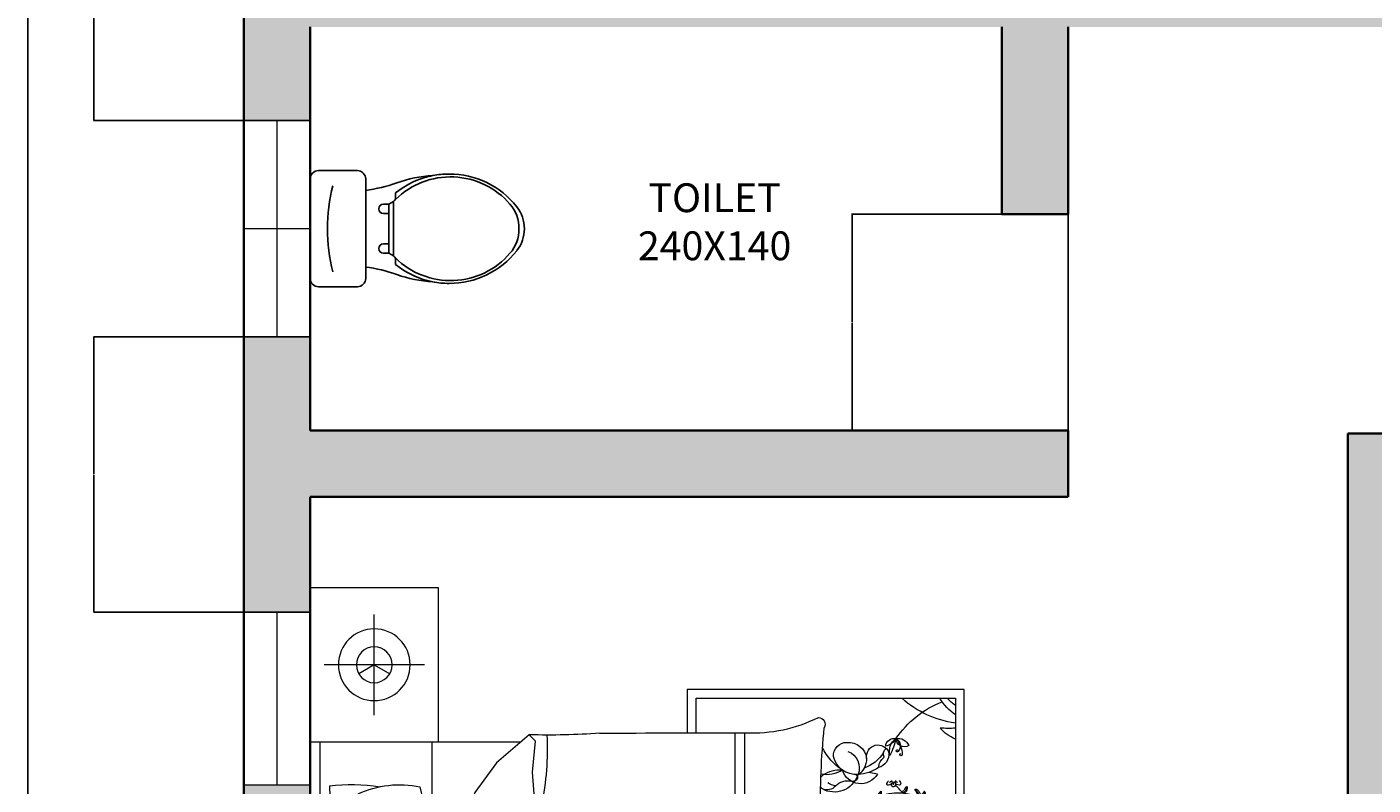
# Model space of a CAD drawing. Units: centimetres. Extents: x 2178 to 3635, y 1064 to 2635.
# Tile 2 of 9: x 2178 to 2645, y 1502 to 1765. Entities that reach past the tile are written whole.
import ezdxf

# ---------------------------------------------------------------- set-up
doc = ezdxf.new("R2010")
doc.units = ezdxf.units.CM
for name, color, linetype, lineweight in [('A-ANNO-DIMS', 2, 'Continuous', 18), ('A-AREA-IDEN', 7, 'Continuous', 18), ('A-DOOR', 32, 'Continuous', 25), ('A-FLOR-FIXT', 42, 'Continuous', 18), ('A-FURN', 42, 'Continuous', 18), ('A-GLAZ', 4, 'Continuous', 18), ('A-WALL', 7, 'Continuous', 35)]:
    doc.layers.add(name, color=color, linetype=linetype, lineweight=lineweight)
doc.layers.add('A-WALL-PATT', color=18, linetype='Continuous', lineweight=13, true_color=0x000000)
doc.layers.add('WC-Detail_dwgmodels.com', color=251, linetype='Continuous')
doc.layers.add('WC-Outline_dwgmodels.com', color=250, linetype='Continuous')
doc.styles.get("Standard").update_dxf_attribs({"font": 'arial.ttf'})
doc.dimstyles.get("Standard").update_dxf_attribs({"dimtxt": 0.18, "dimasz": 0.18, "dimexe": 0.18, "dimexo": 0.0625, "dimgap": 0.09, "dimtad": 0, "dimtih": 1, "dimtoh": 1, "dimdec": 4, "dimzin": 0, "dimdsep": 46, "dimtxsty": 'Standard', "dimcen": 0.09, "dimadec": 0, "dimazin": 0, "dimtfac": 1, "dimtdec": 4, "dimtofl": 0, "dimtmove": 0, "dimatfit": 3, "dimfxl": 1, "dimtolj": 1, "dimtzin": 0, "dimarcsym": 0})

# ---------------------------------------------------------------- blocks, each defined once
blk = doc.blocks.new('bed')
for p, q in [((2798.77, 2937.13), (3098.77, 2937.13)), ((2858.77, 2937.13), (2858.77, 2854.79)), ((2828.77, 2892.53), (2828.77, 2931.73)), ((3038.77, 2933.28), (2858.77, 2933.28)), ((3068.77, 2892.53), (3068.77, 2931.73)), ((2848.37, 2912.13), (2809.17, 2912.13)), ((3049.17, 2912.13), (3088.37, 2912.13)), ((2858.77, 2889.72), (3038.77, 2889.72)), ((2900.44, 2880.8), (2933.16, 2889.72)), ((2941.19, 2889.72), (2924.75, 2866.84)), ((2878.57, 2872.91), (2900.44, 2880.8)), ((2867.02, 2864.41), (2878.57, 2872.91)), ((3037.85, 2874.18), (2928.92, 2872.64)), ((3037.97, 2877.26), (2931.16, 2875.76)), ((2924.75, 2866.84), (2918.06, 2849.23)), ((2856.09, 2851.66), (2867.02, 2864.41)), ((3037.71, 2861.65), (2922.6, 2861.18)), ((3037.69, 2864.73), (2923.78, 2864.28)), ((2858.52, 2849.23), (2856.09, 2851.66)), ((2870.67, 2850.44), (2858.52, 2849.23)), ((2885.86, 2849.23), (2870.67, 2850.44)), ((2899.23, 2847.41), (2885.86, 2849.23)), ((2907.13, 2843.76), (2899.23, 2847.41)), ((2918.06, 2849.23), (2916.85, 2841.33)), ((2916.85, 2841.33), (2907.13, 2843.76)), ((2838.37, 2790.07), (2855.34, 2790.07)), ((2838.37, 2682), (2838.37, 2790.07)), ((3040.44, 2790.07), (3057.08, 2790.07)), ((3057.08, 2790.07), (3057.08, 2682)), ((2855.33, 2786.59), (2841.85, 2786.59)), ((2841.85, 2786.59), (2841.85, 2685.48)), ((3053.6, 2786.59), (3040.38, 2786.59)), ((3053.6, 2685.48), (3053.6, 2786.59)), ((3040.42, 2767.62), (2855.31, 2767.62)), ((3040.13, 2771.36), (2855.32, 2771.36)), ((3009.67, 2738.15), (2887.87, 2738.15)), ((2871.41, 2715.89), (2870.75, 2719.28)), ((2892.38, 2715.89), (2893.04, 2719.28)), ((3003.07, 2715.89), (3002.41, 2719.28)), ((3024.04, 2715.89), (3024.7, 2719.28)), ((2841.85, 2685.48), (3053.6, 2685.48)), ((3057.08, 2682), (2838.37, 2682))]:
    blk.add_line(p, q)
for points in [[(2858.77, 2887.13), (2798.77, 2887.13), (2798.77, 2937.13)], [(3038.77, 2937.13), (3038.77, 2887.13), (3098.77, 2887.13), (3098.77, 2937.13)], [(2828.77, 2912.13), (2832.27, 2918.19)], [(3068.77, 2912.13), (3065.27, 2918.19)], [(2828.77, 2912.13), (2832.27, 2906.07)], [(3068.77, 2912.13), (3065.27, 2906.07)]]:
    blk.add_lwpolyline(points)
for points in [[(2876, 2929.65, 0.074897), (2876.37, 2910.06, -0.472817)], [(2947.37, 2908.96, 0.14099), (2947.97, 2928.95, 0.235245)], [(2960.18, 2908.96, -0.14099), (2959.58, 2928.95, -0.235245)], [(3021.54, 2929.65, -0.074897), (3021.18, 2910.06, 0.472817)], [(2855.46, 2824.19, 0.001242), (2855.31, 2767.26, -0.127202), (2849.3, 2738.9)], [(3040.05, 2773.72, 0.056112), (3042.23, 2757.21, 0.095341), (3046.45, 2741.32)]]:
    blk.add_lwpolyline(points, format="xyb")
for centre, radius in [((2828.77, 2912.13), 14), ((3068.77, 2912.13), 14), ((2828.77, 2912.13), 7), ((3068.77, 2912.13), 7), ((2888.74, 2705.02), 0.764), ((3006.71, 2705.02), 0.764), ((2883.74, 2696.97), 0.764), ((3011.71, 2696.97), 0.764)]:
    blk.add_circle(centre, radius)
for centre, radius, start, end in [((2917.11, 2821.09), 108.8, 82.2196, 99.497), ((2985.93, 2877.16), 52.74, 76.3427, 101.1841), ((3041.36, 5784.66), 2859.79, 266.68521, 267.14978), ((2940.09, 2876.08), 53.46, 81.5249, 103.96), ((2963.69, 2914.69), 14.84, 63.3437, 106.1026), ((2856.18, 5784.66), 2859.79, 272.85022, 273.31479), ((2914.22, 2902.19), 38.67, 155.1316, 191.7583), ((2983.32, 2902.19), 38.67, 348.2417, 24.8684), ((2912, 2898.93), 36.76, 354.0129, 15.8293), ((2995.54, 2898.93), 36.76, 164.1707, 185.9871), ((2886.7, 2933.16), 40.2, 255.1039, 281.0369), ((2907.87, 2961.74), 69.73, 258.0397, 289.2615), ((2936.1, 2946.52), 52.9, 259.8617, 283.6238), ((2965.7, 2909.52), 15.9, 245.0183, 288.5407), ((2993.49, 2930.2), 38.19, 243.8761, 286.1746), ((3010.84, 2933.16), 40.2, 258.9631, 284.8961), ((3576.57, 2853.06), 539.05, 176.1, 180.9282), ((2581.02, 2844.2), 275.17, 355.8294, 1.553), ((2861.22, 2957.89), 113.22, 267.4519, 281.3392), ((2888.28, 2822.94), 24.42, 66.2616, 101.3392), ((2937.68, 2954.7), 116.34, 250.1194, 259.3383), ((2916.17, 2841.09), 0.724, 268.8623, 19.7536), ((3740.68, 2833.46), 703.17, 179.11454, 184.87351), ((3044.17, 2739.79), 2.73, 246.5219, 33.8264), ((2852.06, 2739.09), 2.77, 183.98, 297.3412), ((2884.29, 2425.86), 312.3, 89.3433, 95.6887), ((2850.89, 2717.02), 22.71, 33.6671, 63.2997), ((2881.32, 2730.53), 11.57, 145.785, 184.7304), ((2859.22, 2735.93), 12.43, 328.8218, 9.1554), ((2874.61, 2734.83), 3.61, 120.0293, 142.325), ((2868.85, 2732.7), 9.56, 289.2822, 29.1751), ((2873.09, 2735.54), 4.49, 311.5653, 23.8354), ((2874.61, 2734.83), 3.61, 44.4517, 63.558), ((2894.94, 2732.7), 9.56, 150.8249, 250.7178), ((2890.7, 2735.54), 4.49, 156.1646, 228.4347), ((2889.17, 2734.83), 3.61, 113.229, 135.5483), ((2889.17, 2734.83), 3.61, 37.675, 66.7144), ((2882.46, 2730.53), 11.57, 355.2696, 34.215), ((2904.56, 2735.93), 12.43, 169.7133, 211.1782), ((2912.89, 2717.02), 22.71, 111.4941, 146.3329), ((2982.56, 2717.02), 22.71, 33.6671, 68.5059), ((3012.99, 2730.53), 11.57, 145.785, 184.7304), ((2990.89, 2735.93), 12.43, 328.8218, 10.2867), ((3006.28, 2734.83), 3.61, 113.2856, 142.325), ((3000.51, 2732.7), 9.56, 289.2822, 29.1751), ((3006.28, 2734.83), 3.61, 44.4517, 66.7144), ((3004.75, 2735.54), 4.49, 311.5653, 23.8354), ((3018.86, 2446.37), 291.92, 85.2402, 91.8035), ((3026.6, 2732.7), 9.56, 150.8249, 250.7178), ((3022.36, 2735.54), 4.49, 156.1646, 228.4347), ((3020.84, 2734.83), 3.61, 106.6343, 135.5483), ((3020.84, 2734.83), 3.61, 37.675, 72.5814), ((3014.13, 2730.53), 11.57, 355.2696, 34.215), ((3036.23, 2735.93), 12.43, 169.249, 211.1782), ((3044.56, 2717.02), 22.71, 113.6453, 146.3329), ((2864.12, 2727.92), 5.07, 84.4856, 181.0538), ((2862.56, 2724.18), 9.02, 355.2933, 76.921), ((2880.15, 2727.58), 6.15, 131.5653, 195.1471), ((2867.4, 2730.97), 8.62, 7.436, 29.9149), ((2883.64, 2727.58), 6.15, 344.8529, 48.4347), ((2896.38, 2730.97), 8.62, 150.0851, 172.564), ((2901.22, 2724.18), 9.02, 103.079, 184.7067), ((2899.66, 2727.92), 5.07, 358.9462, 95.5144), ((2995.79, 2727.92), 5.07, 84.4856, 181.0538), ((2994.23, 2724.18), 9.02, 355.2933, 76.921), ((3011.81, 2727.58), 6.15, 131.5653, 195.1471), ((2999.07, 2730.97), 8.62, 7.436, 29.9149), ((3015.3, 2727.58), 6.15, 344.8529, 48.4347), ((3028.05, 2730.97), 8.62, 150.0851, 172.564), ((3032.89, 2724.18), 9.02, 103.079, 184.7067), ((3031.33, 2727.92), 5.07, 358.9462, 95.5144), ((2866.2, 2727.2), 7.17, 174.9449, 262.8857), ((2869.01, 2729.92), 6.96, 201.5819, 291.4221), ((2867.69, 2722.36), 7.46, 299.9085, 73.1337), ((2872.41, 2725.49), 1.86, 257.3041, 15.1471), ((2896.09, 2722.36), 7.46, 106.8663, 240.0915), ((2891.37, 2725.49), 1.86, 164.8529, 282.6959), ((2894.77, 2729.92), 6.96, 248.5779, 338.4181), ((2897.59, 2727.2), 7.17, 277.1143, 5.0551), ((2997.86, 2727.2), 7.17, 174.9449, 262.8857), ((3000.68, 2729.92), 6.96, 201.5819, 291.4221), ((2999.36, 2722.36), 7.46, 299.9085, 73.1337), ((3004.08, 2725.49), 1.86, 257.3041, 15.1471), ((3027.76, 2722.36), 7.46, 106.8663, 240.0915), ((3023.04, 2725.49), 1.86, 164.8529, 282.6959), ((3026.44, 2729.92), 6.96, 248.5779, 338.4181), ((3029.25, 2727.2), 7.17, 277.1143, 5.0551), ((2864.55, 2715.65), 4.5, 80.264, 250.8688), ((2855.62, 2725.56), 14.16, 301.2614, 341.7045), ((2864.95, 2728.79), 8.71, 272.3591, 324.0401), ((2855.49, 2724.42), 16.1, 326.2883, 356.5076), ((2881.32, 2730.53), 11.57, 212.7011, 216.3445), ((2882.75, 2722.67), 0.578, 102.7051, 280.4384), ((2882.69, 2723.02), 0.94, 280.4384, 100.4136), ((2882.46, 2730.53), 11.57, 323.6555, 327.2989), ((2898.83, 2728.79), 8.71, 215.9599, 267.6409), ((2908.3, 2724.42), 16.1, 183.4924, 213.7117), ((2908.16, 2725.56), 14.16, 198.2955, 238.7386), ((2899.24, 2715.65), 4.5, 289.1312, 99.736), ((2951.17, 2718.35), 3.25, 63.0274, 163.8037), ((2947.89, 2725.94), 6.69, 271.4585, 315.3727), ((2954.28, 2718.35), 3.25, 16.1963, 116.9726), ((2957.56, 2725.94), 6.69, 224.6273, 268.5415), ((2996.21, 2715.65), 4.5, 80.264, 250.8688), ((2987.29, 2725.56), 14.16, 301.2614, 341.7045), ((2996.62, 2728.79), 8.71, 272.3591, 324.0401), ((2987.15, 2724.42), 16.1, 326.2883, 356.5076), ((3012.99, 2730.53), 11.57, 212.7011, 216.3445), ((3012.76, 2723.02), 0.94, 79.5864, 259.5616), ((3012.7, 2722.67), 0.578, 259.5616, 77.2949), ((3014.13, 2730.53), 11.57, 323.6555, 327.2989), ((3030.5, 2728.79), 8.71, 215.9599, 267.6409), ((3039.96, 2724.42), 16.1, 183.4924, 213.7117), ((3039.83, 2725.56), 14.16, 198.2955, 238.7386), ((3030.9, 2715.65), 4.5, 289.1312, 99.736), ((2863.47, 2717), 5.62, 265.969, 344.3045), ((2869.52, 2709.53), 5.99, 96.1662, 141.5825), ((2879.44, 2713.73), 1.58, 101.3256, 154.4621), ((2877.17, 2719.07), 4.74, 280.2588, 300.656), ((2903.55, 2707.57), 24.85, 163.5842, 183.8277), ((2876.15, 2719.06), 4.82, 308.2101, 316.3071), ((2879.11, 2715.89), 1.44, 278.3432, 4.2869), ((2878.31, 2717.16), 2.51, 300.656, 332.6341), ((2880.2, 2715.5), 0.611, 55.7657, 157.4417), ((2903.55, 2707.57), 24.85, 153.0032, 159.8941), ((2881.15, 2716.07), 0.611, 84.3784, 186.0543), ((2880.58, 2718.52), 2.51, 269.1859, 301.164), ((2881.32, 2717.22), 1.44, 237.5332, 323.4768), ((2879.92, 2721.32), 4.82, 285.5129, 293.6099), ((2883.07, 2715.9), 1.58, 87.3579, 140.4944), ((2879.43, 2720.42), 4.74, 301.164, 321.5612), ((2875.57, 2721.25), 8.46, 324.6898, 333.4936), ((2894.26, 2709.53), 5.99, 38.4175, 83.8338), ((2900.32, 2717), 5.62, 195.6955, 274.031), ((2951.1, 2680.2), 39.18, 94.4623, 172.255), ((2951.27, 2716.33), 4.34, 137.7873, 219.1145), ((2946.34, 2716.47), 3.27, 298.5391, 58.3627), ((2951.26, 2719.13), 3.2, 177.7585, 283.852), ((2950.61, 2713.61), 6.19, 45.5411, 114.3101), ((2956.25, 2745.4), 27.41, 252.593, 267.2582), ((2957.43, 2722.47), 9.91, 198.9159, 238.011), ((2954.84, 2713.61), 6.19, 65.6899, 134.4589), ((2949.2, 2745.4), 27.41, 272.7418, 287.407), ((2951.92, 2716.43), 0.424, 283.852, 219.9245), ((2952.44, 2714.47), 0.487, 238.011, 71.5592), ((2952.52, 2714.71), 0.236, 71.5592, 188.0167), ((2953.01, 2714.47), 0.487, 108.4408, 301.989), ((2952.93, 2714.71), 0.236, 351.9833, 108.4408), ((2953.49, 2716.59), 0.255, 320.1909, 256.0209), ((2948.02, 2722.47), 9.91, 301.989, 341.0841), ((2954.19, 2719.13), 3.2, 256.148, 2.2415), ((2959.11, 2716.47), 3.27, 121.6373, 241.4609), ((2954.18, 2716.33), 4.34, 320.8855, 42.2127), ((2953.08, 2689.24), 30.32, 352.8636, 81.8197), ((2995.13, 2717), 5.62, 265.969, 344.3045), ((3001.19, 2709.53), 5.99, 96.1662, 141.5825), ((3012.38, 2715.9), 1.58, 39.5056, 92.6421), ((3016.02, 2720.42), 4.74, 218.4388, 238.836), ((3019.88, 2721.25), 8.46, 206.5064, 215.3102), ((3014.13, 2717.22), 1.44, 216.5232, 302.4668), ((3014.87, 2718.52), 2.51, 238.836, 270.8141), ((3015.53, 2721.32), 4.82, 246.3901, 254.4871), ((2991.9, 2707.57), 24.85, 20.1059, 26.9968), ((3014.3, 2716.07), 0.611, 353.9457, 95.6216), ((3016.34, 2715.89), 1.44, 175.7131, 261.6568), ((3015.25, 2715.5), 0.611, 22.5583, 124.2343), ((3017.14, 2717.16), 2.51, 207.3659, 239.344), ((2991.9, 2707.57), 24.85, 356.1723, 16.4158), ((3019.3, 2719.06), 4.82, 223.6929, 231.7899), ((3018.28, 2719.07), 4.74, 239.344, 259.7412), ((3016.01, 2713.73), 1.58, 25.5379, 78.6744), ((3031.98, 2717), 5.62, 195.6955, 274.031), ((3025.93, 2709.53), 5.99, 38.4175, 83.8338), ((2860.73, 2709.42), 3.25, 92.9516, 193.728), ((2854.09, 2714.37), 6.69, 301.3827, 345.2969), ((2862.6, 2705.03), 6.19, 75.4653, 144.2343), ((2851.64, 2735.41), 27.41, 282.5173, 297.1824), ((2863.62, 2710.77), 2.76, 63.9755, 143.2681), ((2874.99, 2710.74), 1.27, 101.5637, 142.6358), ((2873.93, 2709.56), 0.764, 273.2768, 86.7232), ((2874.82, 2710.28), 0.73, 91.1081, 181.8675), ((2875.59, 2708.82), 1.58, 80.3487, 133.6538), ((2873.96, 2711.74), 1.84, 288.7263, 352.5032), ((2875.3, 2707.17), 2.5, 83.0852, 105.7171), ((2875.21, 2711.65), 0.59, 345.2356, 144.9248), ((2875.75, 2709.72), 0.658, 317.6792, 80.3487), ((2878.27, 2722.86), 8.46, 268.3264, 277.1302), ((2900.16, 2710.77), 2.76, 36.7319, 116.0245), ((2901.18, 2705.03), 6.19, 35.7657, 104.5347), ((2912.15, 2735.41), 27.41, 242.8176, 257.4827), ((2903.05, 2709.42), 3.25, 346.272, 87.0484), ((2909.69, 2714.37), 6.69, 194.7031, 238.6173), ((2992.4, 2709.42), 3.25, 92.9516, 193.728), ((2985.76, 2714.37), 6.69, 301.3827, 345.2969), ((2994.27, 2705.03), 6.19, 75.4653, 144.2343), ((2983.3, 2735.41), 27.41, 282.5173, 297.1824), ((2995.29, 2710.77), 2.76, 63.9755, 143.2681), ((3017.18, 2722.86), 8.46, 262.8698, 271.6736), ((3019.7, 2709.72), 0.658, 99.6513, 222.3208), ((3019.86, 2708.82), 1.58, 46.3462, 99.6513), ((3020.24, 2711.65), 0.59, 35.0752, 194.7644), ((3021.49, 2711.74), 1.84, 187.4968, 251.2737), ((3020.15, 2707.17), 2.5, 74.2829, 96.9148), ((3020.63, 2710.28), 0.73, 358.1325, 88.8919), ((3020.46, 2710.74), 1.27, 37.3642, 78.4363), ((3021.52, 2709.56), 0.764, 93.2768, 266.7232), ((3031.83, 2710.77), 2.76, 36.7319, 116.0245), ((3032.85, 2705.03), 6.19, 35.7657, 104.5347), ((3043.81, 2735.41), 27.41, 242.8176, 257.4827), ((3041.36, 2714.37), 6.69, 194.7031, 238.6173), ((3034.72, 2709.42), 3.25, 346.272, 87.0484), ((2812.68, 2680.2), 39.18, 7.745, 41.8856), ((2879.7, 2676.32), 39.18, 124.3865, 158.5908), ((2861.82, 2707.73), 4.34, 167.7115, 249.0387), ((2857.48, 2705.38), 3.27, 328.4633, 88.2869), ((2864.1, 2716.11), 9.91, 228.8402, 267.9352), ((2860.42, 2710.14), 3.2, 207.6827, 313.7762), ((2862.34, 2708.13), 0.424, 313.7762, 249.7183), ((2863.71, 2706.94), 0.236, 101.4834, 217.9409), ((2863.76, 2706.7), 0.487, 267.9352, 101.4834), ((2874.97, 2708.15), 1.26, 217.7621, 259.0403), ((2876.33, 2709.83), 2.32, 203.4276, 227.6104), ((2875.31, 2710.12), 1.25, 229.7889, 317.6792), ((2873.9, 2707.47), 1.78, 355.053, 68.3618), ((2875.09, 2707.37), 0.586, 232.4737, 355.053), ((2857.98, 2686.43), 28.48, 43.1541, 52.0459), ((2877.65, 2703.63), 1.58, 101.3256, 154.4621), ((2875.39, 2708.98), 4.74, 280.2588, 300.656), ((2876.48, 2712.77), 8.46, 268.3264, 277.1302), ((2874.36, 2708.97), 4.82, 308.2101, 316.3071), ((2877.32, 2705.8), 1.44, 278.3432, 4.2869), ((2876.52, 2707.06), 2.51, 300.656, 332.6341), ((2878.41, 2705.4), 0.611, 55.7657, 157.4417), ((2891.17, 2706.94), 12.46, 184.756, 209.2041), ((2909.1, 2733.46), 40.99, 222.2412, 232.1744), ((2884.75, 2705.38), 2.12, 272.8499, 356.1226), ((2882.89, 2706.16), 3.48, 304.5369, 16.3699), ((2883.26, 2704.56), 2.05, 321.7607, 7.9252), ((2887.73, 2705.18), 2.46, 127.3105, 187.9252), ((2884.34, 2705.45), 2.53, 355.0106, 41.658), ((2892.45, 2690.4), 14.94, 113.0501, 113.8477), ((2888.54, 2702.71), 2.41, 104.7558, 148.0499), ((2887.18, 2704.44), 1.51, 247.4086, 351.4386), ((2887.9, 2706.08), 1.04, 126.1046, 271.4281), ((2887.78, 2706.37), 0.749, 353.7526, 131.7054), ((2887.61, 2704.38), 0.506, 262.906, 7.132), ((2887.08, 2705.48), 1.05, 0.0645, 61.1507), ((2887.33, 2706.37), 1.2, 311.8413, 355.7877), ((2889.78, 2703.61), 1.26, 151.2196, 259.0403), ((2889.8, 2706.2), 1.27, 101.5637, 176.365), ((2889.63, 2705.74), 0.73, 91.1081, 181.8675), ((2891.14, 2705.29), 2.32, 203.4276, 227.6104), ((2890.41, 2704.28), 1.58, 80.3487, 133.6538), ((2890.12, 2705.58), 1.25, 229.7889, 317.6792), ((2888.77, 2707.2), 1.84, 288.7263, 352.5032), ((2888.71, 2702.93), 1.78, 355.053, 68.3618), ((2890.11, 2702.63), 2.5, 83.0852, 105.7171), ((2890.02, 2707.11), 0.59, 345.2356, 144.9248), ((2890.56, 2705.18), 0.658, 317.6792, 80.3487), ((2892.45, 2690.4), 14.94, 87.1071, 94.7585), ((2900.02, 2706.7), 0.487, 78.5166, 272.0648), ((2899.68, 2716.11), 9.91, 272.0648, 311.1598), ((2900.07, 2706.94), 0.236, 322.0591, 78.5166), ((2903.37, 2710.14), 3.2, 226.2238, 332.3173), ((2901.49, 2708.3), 0.255, 290.2667, 226.2271), ((2906.3, 2705.38), 3.27, 91.7131, 211.5367), ((2901.96, 2707.73), 4.34, 290.9613, 12.2885), ((2884.08, 2676.32), 39.18, 21.4092, 55.6135), ((3011.37, 2676.32), 39.18, 124.3865, 158.5908), ((2993.49, 2707.73), 4.34, 167.7115, 249.0387), ((2992.08, 2710.14), 3.2, 207.6827, 313.7762), ((2995.76, 2716.11), 9.91, 228.8402, 267.9352), ((2989.15, 2705.38), 3.27, 328.4633, 88.2869), ((2994.01, 2708.13), 0.424, 313.7762, 249.7183), ((2995.38, 2706.94), 0.236, 101.4834, 217.9409), ((2995.43, 2706.7), 0.487, 267.9352, 101.4834), ((3003, 2690.4), 14.94, 85.2415, 92.8929), ((3004.89, 2705.18), 0.658, 99.6513, 222.3208), ((3005.33, 2705.58), 1.25, 222.3208, 310.2111), ((3005.04, 2704.28), 1.58, 46.3462, 99.6513), ((3005.43, 2707.11), 0.59, 35.0752, 194.7644), ((3006.68, 2707.2), 1.84, 187.4968, 251.2737), ((3006.74, 2702.93), 1.78, 111.6382, 184.947), ((3005.34, 2702.63), 2.5, 74.2829, 96.9148), ((3005.82, 2705.74), 0.73, 358.1325, 88.8919), ((3004.31, 2705.29), 2.32, 312.3896, 336.5724), ((3005.65, 2706.2), 1.27, 3.635, 78.4363), ((3005.67, 2703.61), 1.26, 280.9597, 28.7804), ((3008.27, 2704.44), 1.51, 188.5614, 292.5914), ((3007.67, 2706.37), 0.749, 48.2946, 186.2474), ((3008.12, 2706.37), 1.2, 184.2123, 228.1587), ((3008.37, 2705.48), 1.05, 118.8493, 179.9355), ((3007.84, 2704.38), 0.506, 172.868, 277.094), ((3007.55, 2706.08), 1.04, 268.5719, 53.8954), ((3006.91, 2702.71), 2.41, 31.9501, 75.2442), ((3011.11, 2705.45), 2.53, 138.342, 184.9894), ((3010.7, 2705.38), 2.12, 183.8774, 267.1501), ((3003, 2690.4), 14.94, 66.1523, 66.9499), ((3012.56, 2706.16), 3.48, 163.6301, 235.4631), ((3007.72, 2705.18), 2.46, 352.0748, 52.6895), ((3012.19, 2704.56), 2.05, 172.0748, 218.2393), ((2986.35, 2733.46), 40.99, 307.8256, 317.7588), ((3004.28, 2706.94), 12.46, 330.7959, 355.244), ((3037.47, 2686.43), 28.48, 127.9541, 136.8459), ((3017.04, 2705.4), 0.611, 22.5583, 124.2343), ((3018.13, 2705.8), 1.44, 175.7131, 261.6568), ((3018.93, 2707.06), 2.51, 207.3659, 239.344), ((3021.09, 2708.97), 4.82, 223.6929, 231.7899), ((3020.06, 2708.98), 4.74, 239.344, 259.7412), ((3018.97, 2712.77), 8.46, 262.8698, 271.6736), ((3017.8, 2703.63), 1.58, 25.5379, 78.6744), ((3020.14, 2710.12), 1.25, 222.3208, 310.2111), ((3021.55, 2707.47), 1.78, 111.6382, 184.947), ((3020.36, 2707.37), 0.586, 184.947, 307.5263), ((3019.12, 2709.83), 2.32, 312.3896, 336.5724), ((3020.48, 2708.15), 1.26, 280.9597, 322.2379), ((3031.69, 2706.7), 0.487, 78.5166, 272.0648), ((3031.35, 2716.11), 9.91, 272.0648, 311.1598), ((3031.74, 2706.94), 0.236, 322.0591, 78.5166), ((3035.03, 2710.14), 3.2, 226.2238, 332.3173), ((3033.16, 2708.3), 0.255, 290.2667, 226.2271), ((3037.97, 2705.38), 3.27, 91.7131, 211.5367), ((3033.63, 2707.73), 4.34, 290.9613, 12.2885), ((3015.75, 2676.32), 39.18, 21.4092, 55.6135), ((3082.77, 2680.2), 39.18, 138.1144, 172.255), ((2878.18, 2700.87), 0.853, 146.8636, 236.9021), ((2890.21, 2719.66), 22.32, 235.1882, 238.8844), ((2879.65, 2702.11), 2.31, 199.4799, 267.6828), ((2879.39, 2701.23), 1.99, 212.8155, 277.3992), ((2878.23, 2699.91), 2.31, 266.9701, 338.2913), ((2879.13, 2701.31), 0.883, 238.8844, 314.2646), ((2878.94, 2699.33), 1.99, 280.3057, 17.1958), ((2878.77, 2699.13), 0.883, 306.3746, 21.7548), ((2880.21, 2699.7), 0.666, 19.3605, 201.7548), ((2880.22, 2700.2), 0.666, 311.8703, 134.2646), ((2892.74, 2694.13), 13.31, 153.7819, 158.2913), ((2882.15, 2703.22), 3.48, 247.2305, 319.0635), ((2881, 2702.05), 2.05, 264.4544, 310.6188), ((2891.17, 2706.94), 12.46, 214.0033, 222.4917), ((2882.5, 2701.23), 2.12, 218.3208, 298.8162), ((2892.45, 2690.4), 14.94, 120.544, 139.818), ((2882.9, 2698.03), 1.04, 126.1046, 271.4281), ((2882.78, 2698.31), 0.749, 353.7526, 131.7054), ((2883.94, 2698.62), 2.46, 70.0041, 130.6188), ((2882.35, 2701.62), 2.53, 297.7043, 344.3516), ((2884.8, 2698.15), 1.27, 101.5637, 176.365), ((2883.78, 2699.15), 1.84, 288.7263, 352.5032), ((2885.03, 2699.06), 0.59, 345.2356, 144.9248), ((2883.69, 2701.61), 2.05, 8.7227, 54.8872), ((2883.8, 2699.97), 3.48, 0.278, 72.111), ((2885.36, 2701.25), 2.12, 20.5253, 88.5375), ((2888.15, 2702.29), 2.46, 188.7227, 249.3375), ((2887.13, 2703.59), 0.757, 148.0499, 225.6268), ((2884.99, 2701.06), 2.53, 334.9899, 21.6373), ((2889.9, 2702.83), 0.586, 232.4737, 355.053), ((2948.18, 2697.36), 3.25, 63.0274, 163.8037), ((2944.89, 2704.96), 6.69, 271.4585, 315.3727), ((2947.61, 2692.63), 6.19, 45.5411, 114.3101), ((2957.84, 2692.63), 6.19, 65.6899, 134.4589), ((2957.27, 2697.36), 3.25, 16.1963, 116.9726), ((2960.56, 2704.96), 6.69, 224.6273, 268.5415), ((3005.55, 2702.83), 0.586, 184.947, 307.5263), ((3010.46, 2701.06), 2.53, 158.3627, 205.0101), ((3010.09, 2701.25), 2.12, 91.4625, 159.4747), ((3011.65, 2699.97), 3.48, 107.889, 179.722), ((3007.3, 2702.29), 2.46, 290.6625, 351.2773), ((3008.32, 2703.59), 0.757, 314.3732, 31.9501), ((3011.76, 2701.61), 2.05, 125.1128, 171.2773), ((3010.42, 2699.06), 0.59, 35.0752, 194.7644), ((3011.67, 2699.15), 1.84, 187.4968, 251.2737), ((3003, 2690.4), 14.94, 40.182, 59.456), ((3011.51, 2698.62), 2.46, 49.3812, 109.9959), ((3013.3, 2703.22), 3.48, 220.9365, 292.7695), ((3013.1, 2701.62), 2.53, 195.6484, 242.2957), ((3010.65, 2698.15), 1.27, 3.635, 78.4363), ((3012.67, 2698.31), 0.749, 48.2946, 186.2474), ((3012.95, 2701.23), 2.12, 241.1838, 321.6792), ((3012.55, 2698.03), 1.04, 268.5719, 53.8954), ((3014.45, 2702.05), 2.05, 229.3812, 275.5456), ((3004.28, 2706.94), 12.46, 317.5083, 325.9967), ((3016.51, 2699.33), 1.99, 162.8042, 259.6943), ((3015.23, 2700.2), 0.666, 45.7354, 228.1297), ((3015.24, 2699.7), 0.666, 338.2452, 160.6395), ((3002.71, 2694.13), 13.31, 21.7087, 26.2181), ((3017.22, 2699.91), 2.31, 201.7087, 273.0299), ((3016.32, 2701.31), 0.883, 225.7354, 301.1156), ((3016.68, 2699.13), 0.883, 158.2452, 233.6254), ((3016.06, 2701.23), 1.99, 262.6008, 327.1845), ((3015.8, 2702.11), 2.31, 272.3172, 340.5201), ((3005.24, 2719.66), 22.32, 301.1156, 304.8118), ((3017.27, 2700.87), 0.853, 303.0979, 33.1364), ((2866.06, 2716.39), 22.32, 302.6784, 306.3746), ((2878.82, 2698.08), 0.853, 214.3538, 304.3923), ((2882.14, 2695.53), 0.757, 148.0499, 225.6268), ((2883.54, 2694.66), 2.41, 104.7558, 148.0499), ((2882.19, 2696.38), 1.51, 247.4086, 351.4386), ((2882.61, 2696.32), 0.506, 262.906, 7.132), ((2882.08, 2697.42), 1.05, 0.0645, 61.1507), ((2882.33, 2698.32), 1.2, 311.8413, 355.7877), ((2884.78, 2695.55), 1.26, 151.2196, 259.0403), ((2884.63, 2697.69), 0.73, 91.1081, 181.8675), ((2886.15, 2697.23), 2.32, 203.4276, 227.6104), ((2885.41, 2696.22), 1.58, 80.3487, 133.6538), ((2885.13, 2697.53), 1.25, 229.7889, 317.6792), ((2883.72, 2694.88), 1.78, 355.053, 68.3618), ((2885.11, 2694.58), 2.5, 83.0852, 105.7171), ((2884.9, 2694.78), 0.586, 232.4737, 355.053), ((2885.56, 2697.13), 0.658, 317.6792, 80.3487), ((2931.45, 2674.95), 19.09, 91.272, 146.5383), ((2938.32, 2671.39), 23.79, 107.8504, 143.6964), ((2950.82, 2664.7), 35.39, 124.0123, 144.053), ((2948.1, 2659.21), 39.18, 94.4623, 117.4146), ((2948.27, 2695.35), 4.34, 137.7873, 219.1145), ((2943.34, 2695.48), 3.27, 298.5391, 58.3627), ((2948.26, 2698.14), 3.2, 177.7585, 283.852), ((2954.43, 2701.48), 9.91, 198.9159, 238.011), ((2953.26, 2724.42), 27.41, 252.593, 267.2582), ((2948.92, 2695.44), 0.424, 283.852, 219.9245), ((2949.44, 2693.49), 0.487, 238.011, 71.5592), ((2949.52, 2693.73), 0.236, 71.5592, 188.0167), ((2952.19, 2724.42), 27.41, 272.7418, 287.407), ((2956.01, 2693.49), 0.487, 108.4408, 301.989), ((2955.93, 2693.73), 0.236, 351.9833, 108.4408), ((2956.49, 2695.61), 0.255, 320.1909, 256.0209), ((2951.02, 2701.48), 9.91, 301.989, 341.0841), ((2957.19, 2698.14), 3.2, 256.148, 2.2415), ((2962.11, 2695.48), 3.27, 121.6373, 241.4609), ((2957.18, 2695.35), 4.34, 320.8855, 42.2127), ((2957.35, 2659.21), 39.18, 62.5854, 85.5377), ((2957, 2692.01), 17.54, 338.117, 6.6195), ((2973.09, 2687.13), 7.03, 346.3898, 79.0739), ((2967.81, 2688.1), 8.89, 342.8609, 41.9049), ((3009.89, 2697.13), 0.658, 99.6513, 222.3208), ((3010.32, 2697.53), 1.25, 222.3208, 310.2111), ((3010.04, 2696.22), 1.58, 46.3462, 99.6513), ((3011.73, 2694.88), 1.78, 111.6382, 184.947), ((3010.55, 2694.78), 0.586, 184.947, 307.5263), ((3010.34, 2694.58), 2.5, 74.2829, 96.9148), ((3010.82, 2697.69), 0.73, 358.1325, 88.8919), ((3009.3, 2697.23), 2.32, 312.3896, 336.5724), ((3010.67, 2695.55), 1.26, 280.9597, 28.7804), ((3013.26, 2696.38), 1.51, 188.5614, 292.5914), ((3013.12, 2698.32), 1.2, 184.2123, 228.1587), ((3013.37, 2697.42), 1.05, 118.8493, 179.9355), ((3012.84, 2696.32), 0.506, 172.868, 277.094), ((3011.91, 2694.66), 2.41, 31.9501, 75.2442), ((3013.31, 2695.53), 0.757, 314.3732, 31.9501), ((3029.39, 2716.39), 22.32, 233.6254, 237.3216), ((3016.63, 2698.08), 0.853, 235.6077, 325.6462), ((2832.33, 2674.95), 19.09, 33.4617, 60.1116), ((2825.46, 2671.39), 23.79, 36.3036, 46.4814), ((2843.02, 2679.37), 15.93, 22.5547, 48.9546), ((2799.39, 2687.93), 54.2, 357.4081, 3.6519), ((2920.76, 2679.37), 15.93, 131.0454, 157.4453), ((2964.39, 2687.93), 54.2, 176.3481, 182.5919), ((2931.06, 2687.93), 54.2, 357.4081, 3.6519), ((2974.69, 2679.37), 15.93, 22.5547, 48.9546), ((3052.43, 2679.37), 15.93, 131.0454, 157.4453), ((3096.06, 2687.93), 54.2, 176.3481, 182.5919), ((3063.12, 2674.95), 19.09, 119.8884, 146.5383), ((3069.99, 2671.39), 23.79, 133.5186, 143.6964), ((2937.15, 2664.88), 21.54, 73.5431, 107.0202), ((2945.68, 2653.78), 31.85, 94.3787, 95.6357), ((2962.46, 2631.95), 56.92, 109.7217, 109.9028), ((2968.3, 2664.88), 21.54, 72.9798, 106.4569), ((2959.77, 2653.78), 31.85, 84.3643, 85.6213), ((2942.99, 2631.95), 56.92, 70.0972, 70.2783)]:
    blk.add_arc(centre, radius, start, end)
blk = doc.blocks.new('pan')
at = {"layer": 'WC-Detail_dwgmodels.com'}
for p, q in [((2845.98, 2656.18), (2845.98, 2658.01)), ((2849.25, 2658.01), (2849.25, 2656.18)), ((2859.76, 2658.01), (2859.76, 2656.18)), ((2863.04, 2656.18), (2863.04, 2658.01)), ((2844.36, 2653.82), (2842.09, 2653.82)), ((2845.06, 2654.5), (2845.98, 2656.18)), ((2854.51, 2654.5), (2845.06, 2654.5)), ((2849.25, 2656.18), (2845.98, 2656.18)), ((2854.51, 2656.18), (2849.25, 2656.18)), ((2854.51, 2656.18), (2859.76, 2656.18)), ((2854.51, 2654.5), (2863.95, 2654.5)), ((2859.76, 2656.18), (2863.04, 2656.18)), ((2863.95, 2654.5), (2863.04, 2656.18)), ((2864.65, 2653.82), (2866.93, 2653.82))]:
    blk.add_line(p, q, dxfattribs=at)
for centre, radius, start, end in [((2854.54, 2618.37), 59.08, 90.028, 104.6712), ((2854.48, 2618.37), 59.08, 75.3288, 89.972), ((2847.61, 2658.01), 1.64, 0, 180), ((2861.4, 2658.01), 1.64, 0, 180), ((2863.72, 2634.72), 27.2, 135.3828, 229.2681), ((2865.36, 2635.16), 29.83, 141.274, 162.7649), ((2863.72, 2634.72), 27.2, 133.3236, 135.3828), ((2845.29, 2634.72), 27.2, 310.7319, 44.6172), ((2845.29, 2634.72), 27.2, 44.6172, 46.6764), ((2843.66, 2635.16), 29.83, 14.6482, 38.726), ((2865.36, 2635.16), 29.83, 162.7649, 168.8583), ((2843.66, 2635.16), 29.83, 11.1417, 14.6482), ((2854.36, 2623.84), 12.85, 229.2681, 270.6684), ((2854.66, 2623.84), 12.85, 269.3316, 310.7319)]:
    blk.add_arc(centre, radius, start, end, dxfattribs=at)
at = {"layer": 'WC-Outline_dwgmodels.com'}
for p, q in [((2854.51, 2683.42), (2837.26, 2683.42)), ((2871.75, 2683.42), (2854.51, 2683.42)), ((2834.37, 2680.53), (2834.37, 2667.05)), ((2874.65, 2667.05), (2874.65, 2680.53)), ((2837.26, 2664.16), (2841.21, 2664.16)), ((2841.21, 2664.16), (2854.51, 2664.16)), ((2867.8, 2664.16), (2854.51, 2664.16)), ((2867.8, 2664.16), (2871.75, 2664.16))]:
    blk.add_line(p, q, dxfattribs=at)
for centre, radius, start, end in [((2837.26, 2680.53), 2.89, 90, 180), ((2871.75, 2680.53), 2.89, 360, 90), ((2837.26, 2667.05), 2.89, 180, 270), ((2871.75, 2667.05), 2.89, 270, 0), ((2788.54, 2671.16), 53.13, 340.4442, 352.4299), ((2920.47, 2671.16), 53.13, 187.5701, 199.5558), ((2880.9, 2638.36), 44.88, 160.4442, 176.7189), ((2828.12, 2638.36), 44.88, 3.2811, 19.5558), ((2865.36, 2635.16), 29.83, 168.8583, 179.8559), ((2843.66, 2635.16), 29.83, 0.1441, 11.1417), ((2865.36, 2635.16), 29.83, 179.8559, 231.7417), ((2843.66, 2635.16), 29.83, 308.2583, 0.1441), ((2854.51, 2621.4), 12.31, 231.7417, 269.9885), ((2854.5, 2621.4), 12.31, 270.0115, 308.2583)]:
    blk.add_arc(centre, radius, start, end, dxfattribs=at)
blk = doc.blocks.new('WIN-0750-2LT')
for p, q in [((0, 0), (0, 23)), ((37.5, 0), (37.5, 23)), ((75, 0), (75, 23)), ((0, 11.5), (75, 11.5))]:
    blk.add_line(p, q)
blk = doc.blocks.new('WIN-0600')
for p, q in [((0, 60), (23, 60)), ((11.5, 60), (11.5, 0)), ((0, 0), (23, 0))]:
    blk.add_line(p, q)
blk = doc.blocks.new('DOOR-0750')
blk.add_line((0, 0), (75, 0))
blk = doc.blocks.new('*D47')
at = {"layer": 'A-ANNO-DIMS', "color": 0, "lineweight": -2, "transparency": 16777216}
for p, q in [((2511.88, 2559.59), (2178.42, 2559.59)), ((2178.6, 2559.41), (2178.6, 1874.27)), ((2178.6, 1188.77), (2178.6, 1873.91)), ((2253.54, 1188.59), (2178.42, 1188.59))]:
    blk.add_line(p, q, dxfattribs=at)
at = {"layer": 'A-ANNO-DIMS', "color": 0, "transparency": 16777216}
for points in [[(2178.57, 2559.41), (2178.63, 2559.41), (2178.6, 2559.59)], [(2178.57, 1188.77), (2178.63, 1188.77), (2178.6, 1188.59)]]:
    blk.add_solid(points, dxfattribs=at)
at = {"layer": 'Defpoints', "color": 0, "transparency": 16777216}
for p in [(2178.6, 2559.59), (2511.95, 2559.59), (2253.6, 1188.59)]:
    blk.add_point(p, dxfattribs=at)
at = {"layer": 'A-ANNO-DIMS', "color": 0, "transparency": 16777216, "insert": (2178.6, 1874.09), "char_height": 0.18, "attachment_point": 5}
blk.add_mtext('\\A1;1371', dxfattribs=at)
blk = doc.blocks.new('*D65')
at = {"layer": 'A-ANNO-DIMS', "color": 0, "lineweight": -2, "transparency": 16777216}
for p, q in [((2539.54, 1699.59), (2464.42, 1699.59)), ((2464.6, 1699.41), (2464.6, 1662.27)), ((2464.6, 1624.77), (2464.6, 1661.91)), ((2539.54, 1624.59), (2464.42, 1624.59))]:
    blk.add_line(p, q, dxfattribs=at)
at = {"layer": 'A-ANNO-DIMS', "color": 0, "transparency": 16777216}
for points in [[(2464.57, 1699.41), (2464.63, 1699.41), (2464.6, 1699.59)], [(2464.57, 1624.77), (2464.63, 1624.77), (2464.6, 1624.59)]]:
    blk.add_solid(points, dxfattribs=at)
at = {"layer": 'Defpoints', "color": 0, "transparency": 16777216}
for p in [(2464.6, 1699.59), (2539.6, 1699.59), (2539.6, 1624.59)]:
    blk.add_point(p, dxfattribs=at)
at = {"layer": 'A-ANNO-DIMS', "color": 0, "transparency": 16777216, "insert": (2464.6, 1662.09), "char_height": 0.18, "attachment_point": 5}
blk.add_mtext('\\A1;75', dxfattribs=at)
blk = doc.blocks.new('*D71')
at = {"layer": 'A-ANNO-DIMS', "color": 0, "lineweight": -2, "transparency": 16777216}
for p, q in [((2276.54, 1657.09), (2201.42, 1657.09)), ((2201.6, 1656.91), (2201.6, 1609.52)), ((2201.6, 1561.77), (2201.6, 1609.16)), ((2276.54, 1561.59), (2201.42, 1561.59))]:
    blk.add_line(p, q, dxfattribs=at)
at = {"layer": 'A-ANNO-DIMS', "color": 0, "transparency": 16777216}
for points in [[(2201.57, 1656.91), (2201.63, 1656.91), (2201.6, 1657.09)], [(2201.57, 1561.77), (2201.63, 1561.77), (2201.6, 1561.59)]]:
    blk.add_solid(points, dxfattribs=at)
at = {"layer": 'Defpoints', "color": 0, "transparency": 16777216}
for p in [(2201.6, 1657.09), (2276.6, 1657.09), (2276.6, 1561.59)]:
    blk.add_point(p, dxfattribs=at)
at = {"layer": 'A-ANNO-DIMS', "color": 0, "transparency": 16777216, "insert": (2201.6, 1609.34), "char_height": 0.18, "attachment_point": 5}
blk.add_mtext('\\A1;95.5', dxfattribs=at)
blk = doc.blocks.new('*D72')
at = {"layer": 'A-ANNO-DIMS', "color": 0, "lineweight": -2, "transparency": 16777216}
for p, q in [((2276.54, 1860.59), (2201.42, 1860.59)), ((2201.6, 1860.41), (2201.6, 1796.52)), ((2201.6, 1732.27), (2201.6, 1796.16)), ((2276.54, 1732.09), (2201.42, 1732.09))]:
    blk.add_line(p, q, dxfattribs=at)
at = {"layer": 'A-ANNO-DIMS', "color": 0, "transparency": 16777216}
for points in [[(2201.57, 1860.41), (2201.63, 1860.41), (2201.6, 1860.59)], [(2201.57, 1732.27), (2201.63, 1732.27), (2201.6, 1732.09)]]:
    blk.add_solid(points, dxfattribs=at)
at = {"layer": 'Defpoints', "color": 0, "transparency": 16777216}
for p in [(2201.6, 1860.59), (2276.6, 1860.59), (2276.6, 1732.09)]:
    blk.add_point(p, dxfattribs=at)
at = {"layer": 'A-ANNO-DIMS', "color": 0, "transparency": 16777216, "insert": (2201.6, 1796.34), "char_height": 0.18, "attachment_point": 5}
blk.add_mtext('\\A1;128.5', dxfattribs=at)

msp = doc.modelspace()

# ---------------------------------------------------------------- hatches: boundary and pattern name
at = {"layer": 'A-WALL-PATT'}
h = msp.add_hatch(color=256, dxfattribs=at)
h.dxf.hatch_style = 1
h.paths.add_polyline_path([(2276.605, 2499.59), (2253.605, 2499.59), (2253.605, 2476.59), (2276.605, 2476.59)])
h.paths.add_polyline_path([(2411.605, 2350.59), (2253.605, 2350.59), (2253.605, 2327.59), (2411.605, 2327.59)])
h.paths.add_polyline_path([(2276.605, 2252.59), (2253.605, 2252.59), (2253.605, 2020.59), (2276.605, 2020.59), (2276.605, 2093.59), (2561.605, 2093.59), (2561.605, 2116.59), (2276.605, 2116.59)])
h.paths.add_polyline_path([(2659.605, 1787.59), (2610.616, 1787.59), (2276.605, 1787.59), (2276.605, 1860.59), (2253.605, 1860.59), (2253.605, 1732.09), (2276.605, 1732.09), (2276.605, 1764.59), (2516.605, 1764.59), (2516.605, 1699.59), (2539.605, 1699.59), (2539.605, 1764.59), (2659.605, 1764.59)])
h.paths.add_polyline_path([(2539.605, 1624.59), (2276.605, 1624.59), (2276.605, 1657.09), (2253.605, 1657.09), (2253.605, 1561.59), (2276.605, 1561.59), (2276.605, 1601.59), (2539.605, 1601.59)])
h.paths.add_polyline_path([(2276.605, 1501.59), (2253.605, 1501.59), (2253.605, 1371.59), (2276.605, 1371.59)])
h.paths.add_polyline_path([(2376.605, 1271.59), (2276.605, 1271.59), (2276.605, 1311.59), (2253.605, 1311.59), (2253.605, 1248.59), (2376.605, 1248.59)])
h.paths.add_polyline_path([(2636.605, 1271.59), (2536.605, 1271.59), (2536.605, 1248.59), (2636.605, 1248.59)])
h.paths.add_polyline_path([(2659.605, 1600.59), (2919.605, 1600.59), (2919.605, 1623.59), (2636.605, 1623.59), (2636.605, 1188.59), (2659.605, 1188.59)])
h.paths.add_polyline_path([(2939.605, 1211.59), (2759.605, 1211.59), (2759.605, 1188.59), (2939.605, 1188.59)])
h.paths.add_polyline_path([(3062.605, 1288.59), (3039.605, 1288.59), (3039.605, 1188.59), (3062.605, 1188.59)])
h.paths.add_polyline_path([(3372.605, 1248.59), (3062.605, 1248.59), (3062.605, 1218.59), (3372.605, 1218.59)])
h.paths.add_polyline_path([(3395.605, 1271.59), (3372.605, 1271.59), (3372.605, 1248.59), (3395.605, 1248.59)])
h.paths.add_polyline_path([(3559.605, 1271.59), (3536.605, 1271.59), (3536.605, 1248.59), (3559.605, 1248.59)])
h.paths.add_polyline_path([(3559.605, 1623.59), (3536.605, 1623.59), (3536.605, 1600.59), (3559.605, 1600.59)])
h.paths.add_polyline_path([(3395.605, 1623.59), (3162.605, 1623.59), (3162.605, 1600.59), (3395.605, 1600.59)])
h.paths.add_polyline_path([(3395.605, 1411.59), (3277.1, 1411.59), (3277.1, 1388.59), (3395.605, 1388.59)])
h.paths.add_polyline_path([(3157.1, 1411.59), (3062.605, 1411.59), (3062.605, 1623.59), (3039.605, 1623.59), (3039.605, 1388.59), (3157.1, 1388.59)])
h.paths.add_polyline_path([(3559.605, 1797.09), (3536.605, 1797.09), (3536.605, 1764.59), (3316.605, 1764.59), (3316.605, 1927.59), (3293.605, 1927.59), (3293.605, 1741.59), (3372.605, 1741.59), (3395.605, 1741.59), (3559.605, 1741.59)])
h.paths.add_polyline_path([(3559.605, 1990.59), (3536.605, 1990.59), (3536.605, 1974.446), (3536.605, 1927.59), (3391.605, 1927.59), (3391.605, 1904.59), (3536.605, 1904.59), (3536.605, 1872.09), (3559.605, 1872.09)])
h.paths.add_polyline_path([(3559.605, 2180.59), (3536.605, 2180.59), (3536.605, 2050.59), (3559.605, 2050.59)])
h.paths.add_polyline_path([(3559.605, 2326.59), (3446.105, 2326.59), (3446.105, 2303.59), (3536.605, 2303.59), (3536.605, 2240.59), (3559.605, 2240.59)])
h.paths.add_polyline_path([(3286.105, 2326.59), (3195.605, 2326.59), (3195.605, 2499.59), (3082.605, 2499.59), (3082.605, 2476.59), (3172.605, 2476.59), (3172.605, 2116.59), (2809.605, 2116.59), (2809.605, 2093.59), (3172.605, 2093.59), (3172.605, 1904.59), (3195.605, 1904.59), (3195.605, 2303.59), (3286.105, 2303.59)])
h.paths.add_polyline_path([(2832.605, 2236.59), (2659.605, 2236.59), (2659.605, 2476.59), (2697.105, 2476.59), (2697.105, 2499.59), (2636.605, 2499.59), (2636.605, 2093.59), (2699.605, 2093.59), (2699.605, 2116.59), (2659.605, 2116.59), (2659.605, 2213.59), (2832.605, 2213.59)])
h.paths.add_polyline_path([(2832.605, 2476.59), (2922.605, 2476.59), (2922.605, 2499.59), (2772.105, 2499.59), (2772.105, 2476.59), (2809.605, 2476.59), (2809.605, 2311.59), (2832.605, 2311.59)])

# ---------------------------------------------------------------- linework, layer by layer
at = {"layer": 'A-WALL'}
for p, q in [((2253.605, 2499.59), (2253.605, 1188.59)), ((2276.605, 1764.59), (2276.605, 1624.59)), ((2516.605, 1764.59), (2516.605, 1699.59)), ((2539.605, 1764.59), (2539.605, 1699.59)), ((2516.605, 1699.59), (2539.605, 1699.59)), ((2276.605, 1624.59), (2539.605, 1624.59)), ((2539.605, 1624.59), (2539.605, 1601.59)), ((2636.605, 1623.59), (2636.605, 1188.59)), ((2636.605, 1623.59), (2919.605, 1623.59)), ((2276.605, 1601.59), (2539.605, 1601.59)), ((2276.605, 1601.59), (2276.605, 1271.59))]:
    msp.add_line(p, q, dxfattribs=at)

# ---------------------------------------------------------------- block references
at = {"layer": 'A-DOOR', "rotation": 270.0000000000007}
msp.add_blockref('DOOR-0750', (2539.605, 1699.59), dxfattribs=at)
at = {"layer": 'A-FLOR-FIXT', "xscale": -1, "rotation": 90}
msp.add_blockref('pan', (4960.024, 4549.097), dxfattribs=at)
at = {"layer": 'A-FURN', "xscale": -0.8894661318613604, "yscale": 0.8894661318613604, "zscale": 0.8894661318613604, "rotation": 90}
msp.add_blockref('bed', (4889.082, 4059.422), dxfattribs=at)
at = {"layer": 'A-GLAZ'}
for name, p, rotation in [('WIN-0750-2LT', (2276.605, 1657.09), 90.0000000000004), ('WIN-0600', (2276.605, 1561.59), 180)]:
    msp.add_blockref(name, p, dxfattribs=dict(at, rotation=rotation))

# ---------------------------------------------------------------- texts
at = {"layer": 'A-AREA-IDEN', "insert": (2361.128, 1710.333), "char_height": 10, "attachment_point": 1}
msp.add_mtext_dynamic_manual_height_columns('\\pxqc;TOILET\\P240X140', width=111.5542, gutter_width=12.5, heights=[0], dxfattribs=at)

# ---------------------------------------------------------------- dimensions: what is measured, and where the dimension line sits
at = {"layer": 'A-ANNO-DIMS'}
for base, p1, p2, override, picture, middle in [((2178.605, 2559.59), (2253.605, 1188.59), (2511.946, 2559.59), {"dimdec": 0, "dimlfac": 1, "dimrnd": 0, "dimzin": 0, "dimdsep": 46, "dimlunit": 2}, '*D47', (2178.605, 1874.09)), ((2201.605, 1860.59), (2276.605, 1732.09), (2276.605, 1860.59), {"dimdec": 1, "dimlfac": 1, "dimrnd": 0, "dimzin": 0, "dimdsep": 46, "dimlunit": 2}, '*D72', (2201.605, 1796.34)), ((2464.605, 1699.59), (2539.605, 1624.59), (2539.605, 1699.59), {"dimdec": 0, "dimlfac": 1, "dimrnd": 0, "dimzin": 0, "dimdsep": 46, "dimlunit": 2}, '*D65', (2464.605, 1662.09)), ((2201.605, 1657.09), (2276.605, 1561.59), (2276.605, 1657.09), {"dimdec": 1, "dimlfac": 1, "dimrnd": 0, "dimzin": 0, "dimdsep": 46, "dimlunit": 2}, '*D71', (2201.605, 1609.34))]:
    dim = msp.add_linear_dim(base=base, p1=p1, p2=p2, angle=90, dimstyle='Standard', override=override, dxfattribs=at)
    dim.commit()
    dim.dimension.update_dxf_attribs({"geometry": picture, "text_midpoint": middle})

doc.saveas('drawing.dxf')
